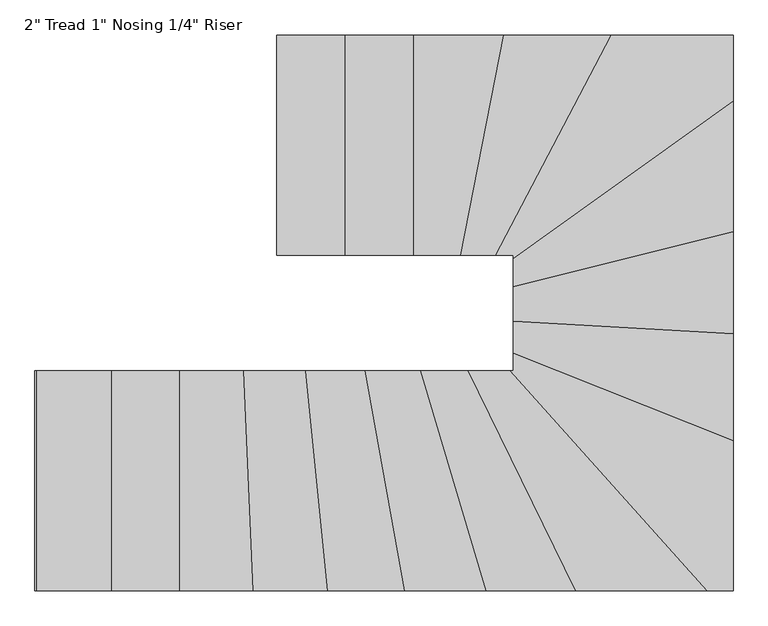
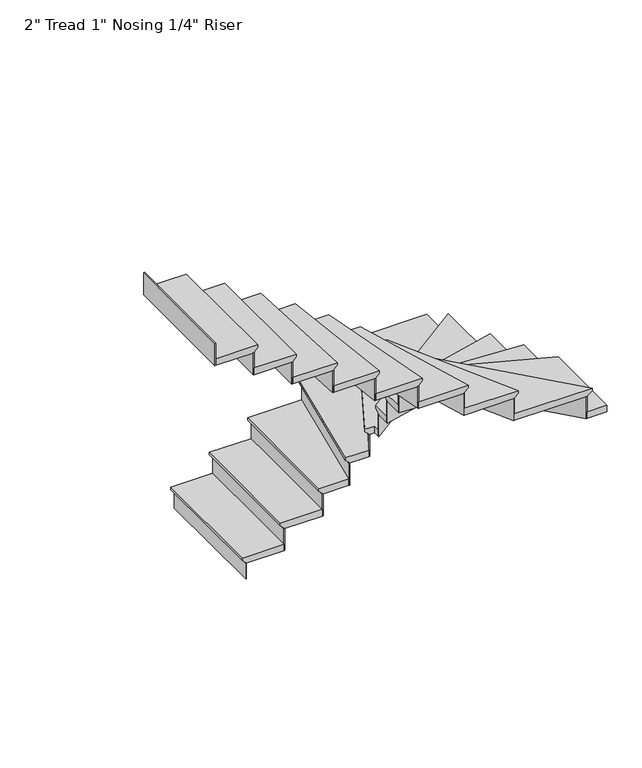
"""IFC4 building model written with IfcOpenShell, lengths in millimetres: stair flight geometry."""

from ifc_helpers import new_model, si_unit, origin, place, context, project, spatial, faceted_brep, source, transform, mapped, element, save


def stair_flight_f84afbbd(model_context):
    return source(origin(), model_context, "Body", "Brep", [
        faceted_brep([(158.6923968, 2024.0935985, 150.2833333), (158.6923968, 2024.0935985, 169.3333333), (158.6923968, 2922.8476133, 169.3333333), (158.6923968, 2922.8476133, 150.2833333), (184.0923968, 2024.0935985, 124.8833333), (184.0923968, 2922.8476133, 124.8833333), (463.4923968, 2024.0935985, 169.3333333), (463.4923968, 2922.8476133, 169.3333333), (184.0923968, 2922.8476133, 118.5333333), (463.4923968, 2922.8476133, 118.5333333), (463.4923968, 2024.0935985, 118.5333333), (184.0923968, 2024.0935985, 118.5333333)], [[[0, 1, 2, 3]], [[4, 0, 3, 5]], [[2, 1, 6, 7]], [[8, 9, 10, 11]], [[2, 7, 9, 8, 5, 3]], [[8, 11, 4, 5]], [[6, 1, 0, 4, 11, 10]], [[7, 6, 10, 9]]]),
        faceted_brep([(184.0923968, 2024.0935985, 118.5333333), (184.0923968, 2024.0935985, 0.0), (190.4423968, 2024.0935985, 0.0), (190.4423968, 2024.0935985, 118.5333333), (184.0923968, 2922.8476133, 118.5333333), (190.4423968, 2922.8476133, 118.5333333), (190.4423968, 2922.8476133, 0.0), (184.0923968, 2922.8476133, 0.0)], [[[0, 1, 2, 3]], [[4, 5, 6, 7]], [[1, 0, 4, 7]], [[2, 1, 7, 6]], [[3, 2, 6, 5]], [[0, 3, 5, 4]]]),
        faceted_brep([(463.4923968, 2024.0935985, 287.8666667), (463.4923968, 2024.0935985, 118.5333333), (469.8423968, 2024.0935985, 118.5333333), (469.8423968, 2024.0935985, 287.8666667), (463.4923968, 2922.8476133, 287.8666667), (469.8423968, 2922.8476133, 287.8666667), (469.8423968, 2922.8476133, 118.5333333), (463.4923968, 2922.8476133, 118.5333333)], [[[0, 1, 2, 3]], [[4, 5, 6, 7]], [[1, 0, 4, 7]], [[2, 1, 7, 6]], [[3, 2, 6, 5]], [[0, 3, 5, 4]]]),
        faceted_brep([(438.0923968, 2922.8476133, 338.6666667), (438.0923968, 2024.0935985, 338.6666667), (742.8923968, 2024.0935985, 338.6666667), (742.8923968, 2922.8476133, 338.6666667), (463.4923968, 2922.8476133, 287.8666667), (742.8923968, 2922.8476133, 287.8666667), (742.8923968, 2024.0935985, 287.8666667), (463.4923968, 2024.0935985, 287.8666667), (463.4923968, 2922.8476133, 294.2166667), (438.0923968, 2922.8476133, 319.6166667), (463.4923968, 2024.0935985, 294.2166667), (438.0923968, 2024.0935985, 319.6166667)], [[[0, 1, 2, 3]], [[4, 5, 6, 7]], [[0, 3, 5, 4, 8, 9]], [[4, 7, 10, 8]], [[2, 1, 11, 10, 7, 6]], [[3, 2, 6, 5]], [[11, 1, 0, 9]], [[10, 11, 9, 8]]]),
        faceted_brep([(742.8923968, 2024.0935985, 457.2), (742.8923968, 2024.0935985, 287.8666667), (749.2423968, 2024.0935985, 287.8666667), (749.2423968, 2024.0935985, 457.2), (742.8923968, 2922.8476133, 457.2), (749.2423968, 2922.8476133, 457.2), (749.2423968, 2922.8476133, 287.8666667), (742.8923968, 2922.8476133, 287.8666667)], [[[0, 1, 2, 3]], [[4, 5, 6, 7]], [[1, 0, 4, 7]], [[2, 1, 7, 6]], [[3, 2, 6, 5]], [[0, 3, 5, 4]]]),
        faceted_brep([(717.4923968, 2922.8476133, 508.0), (717.4923968, 2024.0935985, 508.0), (934.4682952, 2024.0935985, 508.0), (1111.0881205, 2922.8476133, 508.0), (742.8923968, 2922.8476133, 457.2), (1111.0881205, 2922.8476133, 457.2), (934.4682952, 2024.0935985, 457.2), (742.8923968, 2024.0935985, 457.2), (742.8923968, 2922.8476133, 463.55), (717.4923968, 2922.8476133, 488.95), (742.8923968, 2024.0935985, 463.55), (717.4923968, 2024.0935985, 488.95)], [[[0, 1, 2, 3]], [[4, 5, 6, 7]], [[0, 3, 5, 4, 8, 9]], [[4, 7, 10, 8]], [[2, 1, 11, 10, 7, 6]], [[3, 2, 6, 5]], [[11, 1, 0, 9]], [[10, 11, 9, 8]]]),
        faceted_brep([(934.4682952, 2024.0935985, 626.5333333), (934.4682952, 2024.0935985, 457.2), (940.939748, 2024.0935985, 457.2), (940.939748, 2024.0935985, 626.5333333), (1111.0881205, 2922.8476133, 626.5333333), (1117.5595733, 2922.8476133, 626.5333333), (1117.5595733, 2922.8476133, 457.2), (1111.0881205, 2922.8476133, 457.2)], [[[0, 1, 2, 3]], [[4, 5, 6, 7]], [[1, 0, 4, 7]], [[2, 1, 7, 6]], [[3, 2, 6, 5]], [[0, 3, 5, 4]]]),
        faceted_brep([(1085.2023094, 2922.8476133, 677.3333333), (908.5824841, 2024.0935985, 677.3333333), (1081.601446, 2024.0935985, 677.3333333), (1553.5566487, 2922.8476133, 677.3333333), (1111.0881205, 2922.8476133, 626.5333333), (1553.5566487, 2922.8476133, 626.5333333), (1081.601446, 2024.0935985, 626.5333333), (934.4682952, 2024.0935985, 626.5333333), (1111.0881205, 2922.8476133, 632.8833333), (1085.2023094, 2922.8476133, 658.2833333), (934.4682952, 2024.0935985, 632.8833333), (908.5824841, 2024.0935985, 658.2833333)], [[[0, 1, 2, 3]], [[4, 5, 6, 7]], [[0, 3, 5, 4, 8, 9]], [[4, 7, 10, 8]], [[2, 1, 11, 10, 7, 6]], [[3, 2, 6, 5]], [[11, 1, 0, 9]], [[10, 11, 9, 8]]]),
        faceted_brep([(1081.601446, 2024.0935985, 795.8666667), (1081.601446, 2024.0935985, 626.5333333), (1088.7737218, 2024.0935985, 626.5333333), (1088.7737218, 2024.0935985, 795.8666667), (1553.5566487, 2922.8476133, 795.8666667), (1560.7289245, 2922.8476133, 795.8666667), (1560.7289245, 2922.8476133, 626.5333333), (1553.5566487, 2922.8476133, 626.5333333)], [[[0, 1, 2, 3]], [[4, 5, 6, 7]], [[1, 0, 4, 7]], [[2, 1, 7, 6]], [[3, 2, 6, 5]], [[0, 3, 5, 4]]]),
        faceted_brep([(2022.1441983, 2621.1058304, 846.6666667), (2022.1441983, 2922.8476133, 846.6666667), (1524.8675453, 2922.8476133, 846.6666667), (1052.9123426, 2024.0935985, 846.6666667), (1123.3901835, 2024.0935985, 846.6666667), (1123.3901835, 1978.1363323, 846.6666667), (2022.1441983, 2922.8476133, 795.8666667), (2022.1441983, 2621.1058304, 795.8666667), (1123.3901835, 1978.1363323, 795.8666667), (1123.3901835, 2024.0935985, 795.8666667), (1081.601446, 2024.0935985, 795.8666667), (1553.5566487, 2922.8476133, 795.8666667), (1081.601446, 2024.0935985, 802.2166667), (1553.5566487, 2922.8476133, 802.2166667), (1052.9123426, 2024.0935985, 827.6166667), (1524.8675453, 2922.8476133, 827.6166667)], [[[0, 1, 2, 3, 4, 5]], [[6, 7, 8, 9, 10, 11]], [[1, 0, 7, 6]], [[11, 10, 12, 13]], [[4, 3, 14, 12, 10, 9]], [[0, 5, 8, 7]], [[14, 3, 2, 15]], [[12, 14, 15, 13]], [[5, 4, 9, 8]], [[2, 1, 6, 11, 13, 15]]]),
        faceted_brep([(1123.3901835, 1978.1363323, 965.2), (1123.3901835, 1978.1363323, 795.8666667), (1123.3901835, 1970.328676, 795.8666667), (1123.3901835, 1970.328676, 965.2), (2022.1441983, 2621.1058304, 965.2), (2022.1441983, 2613.298174, 965.2), (2022.1441983, 2613.298174, 795.8666667), (2022.1441983, 2621.1058304, 795.8666667)], [[[0, 1, 2, 3]], [[4, 5, 6, 7]], [[1, 0, 4, 7]], [[2, 1, 7, 6]], [[3, 2, 6, 5]], [[0, 3, 5, 4]]]),
        faceted_brep([(2022.1441983, 2652.3364556, 1016.0), (1123.3901835, 2009.3669576, 1016.0), (1123.3901835, 1868.1880985, 1016.0), (2022.1441983, 2093.75794, 1016.0), (2022.1441983, 2621.1058304, 965.2), (2022.1441983, 2093.75794, 965.2), (1123.3901835, 1868.1880985, 965.2), (1123.3901835, 1978.1363323, 965.2), (2022.1441983, 2621.1058304, 971.55), (2022.1441983, 2652.3364556, 996.95), (1123.3901835, 1978.1363323, 971.55), (1123.3901835, 2009.3669576, 996.95)], [[[0, 1, 2, 3]], [[4, 5, 6, 7]], [[0, 3, 5, 4, 8, 9]], [[4, 7, 10, 8]], [[2, 1, 11, 10, 7, 6]], [[3, 2, 6, 5]], [[11, 1, 0, 9]], [[10, 11, 9, 8]]]),
        faceted_brep([(1123.3901835, 1868.1880985, 1134.5333333), (1123.3901835, 1868.1880985, 965.2), (1123.3901835, 1861.6411553, 965.2), (1123.3901835, 1861.6411553, 1134.5333333), (2022.1441983, 2093.75794, 1134.5333333), (2022.1441983, 2087.2109968, 1134.5333333), (2022.1441983, 2087.2109968, 965.2), (2022.1441983, 2093.75794, 965.2)], [[[0, 1, 2, 3]], [[4, 5, 6, 7]], [[1, 0, 4, 7]], [[2, 1, 7, 6]], [[3, 2, 6, 5]], [[0, 3, 5, 4]]]),
        faceted_brep([(2022.1441983, 2119.9457129, 1185.3333333), (1123.3901835, 1894.3758714, 1185.3333333), (1123.3901835, 1727.7101185, 1185.3333333), (2022.1441983, 1676.930447, 1185.3333333), (2022.1441983, 2093.75794, 1134.5333333), (2022.1441983, 1676.930447, 1134.5333333), (1123.3901835, 1727.7101185, 1134.5333333), (1123.3901835, 1868.1880985, 1134.5333333), (2022.1441983, 2093.75794, 1140.8833333), (2022.1441983, 2119.9457129, 1166.2833333), (1123.3901835, 1868.1880985, 1140.8833333), (1123.3901835, 1894.3758714, 1166.2833333)], [[[0, 1, 2, 3]], [[4, 5, 6, 7]], [[0, 3, 5, 4, 8, 9]], [[4, 7, 10, 8]], [[2, 1, 11, 10, 7, 6]], [[3, 2, 6, 5]], [[11, 1, 0, 9]], [[10, 11, 9, 8]]]),
        faceted_brep([(1123.3901835, 1727.7101185, 1303.8666667), (1123.3901835, 1727.7101185, 1134.5333333), (1123.3901835, 1721.3499912, 1134.5333333), (1123.3901835, 1721.3499912, 1303.8666667), (2022.1441983, 1676.930447, 1303.8666667), (2022.1441983, 1670.5703197, 1303.8666667), (2022.1441983, 1670.5703197, 1134.5333333), (2022.1441983, 1676.930447, 1134.5333333)], [[[0, 1, 2, 3]], [[4, 5, 6, 7]], [[1, 0, 4, 7]], [[2, 1, 7, 6]], [[3, 2, 6, 5]], [[0, 3, 5, 4]]]),
        faceted_brep([(2022.1441983, 1702.3709564, 1354.6666667), (1123.3901835, 1753.1506279, 1354.6666667), (1123.3901835, 1594.7393557, 1354.6666667), (2022.1441983, 1238.4229709, 1354.6666667), (2022.1441983, 1676.930447, 1303.8666667), (2022.1441983, 1238.4229709, 1303.8666667), (1123.3901835, 1594.7393557, 1303.8666667), (1123.3901835, 1727.7101185, 1303.8666667), (2022.1441983, 1676.930447, 1310.2166667), (2022.1441983, 1702.3709564, 1335.6166667), (1123.3901835, 1727.7101185, 1310.2166667), (1123.3901835, 1753.1506279, 1335.6166667)], [[[0, 1, 2, 3]], [[4, 5, 6, 7]], [[0, 3, 5, 4, 8, 9]], [[4, 7, 10, 8]], [[3, 2, 6, 5]], [[11, 1, 0, 9]], [[10, 11, 9, 8]], [[2, 1, 11, 10, 7, 6]]]),
        faceted_brep([(1123.3901835, 1594.7393557, 1473.2), (1123.3901835, 1594.7393557, 1303.8666667), (1123.3901835, 1587.9085225, 1303.8666667), (1123.3901835, 1587.9085225, 1473.2), (2022.1441983, 1238.4229709, 1473.2), (2022.1441983, 1231.5921376, 1473.2), (2022.1441983, 1231.5921376, 1303.8666667), (2022.1441983, 1238.4229709, 1303.8666667)], [[[0, 1, 2, 3]], [[4, 5, 6, 7]], [[1, 0, 4, 7]], [[2, 1, 7, 6]], [[3, 2, 6, 5]], [[0, 3, 5, 4]]]),
        faceted_brep([(1880.1651285, 652.4935985, 1524.0), (2022.1441983, 652.4935985, 1524.0), (2022.1441983, 1265.7463038, 1524.0), (1123.3901835, 1622.0626887, 1524.0), (1123.3901835, 1551.2476133, 1524.0), (1076.3040211, 1551.2476133, 1524.0), (2022.1441983, 652.4935985, 1473.2), (1880.1651285, 652.4935985, 1473.2), (1076.3040211, 1551.2476133, 1473.2), (1123.3901835, 1551.2476133, 1473.2), (1123.3901835, 1594.7393557, 1473.2), (2022.1441983, 1238.4229709, 1473.2), (1123.3901835, 1594.7393557, 1479.55), (2022.1441983, 1238.4229709, 1479.55), (1123.3901835, 1622.0626887, 1504.95), (2022.1441983, 1265.7463038, 1504.95)], [[[0, 1, 2, 3, 4, 5]], [[6, 7, 8, 9, 10, 11]], [[1, 0, 7, 6]], [[11, 10, 12, 13]], [[4, 3, 14, 12, 10, 9]], [[0, 5, 8, 7]], [[14, 3, 2, 15]], [[12, 14, 15, 13]], [[2, 1, 6, 11, 13, 15]], [[5, 4, 9, 8]]]),
        faceted_brep([(1076.3040211, 1551.2476133, 1642.5333333), (1076.3040211, 1551.2476133, 1473.2), (1067.7846442, 1551.2476133, 1473.2), (1067.7846442, 1551.2476133, 1642.5333333), (1880.1651285, 652.4935985, 1642.5333333), (1871.6457515, 652.4935985, 1642.5333333), (1871.6457515, 652.4935985, 1473.2), (1880.1651285, 652.4935985, 1473.2)], [[[0, 1, 2, 3]], [[4, 5, 6, 7]], [[1, 0, 4, 7]], [[2, 1, 7, 6]], [[3, 2, 6, 5]], [[0, 3, 5, 4]]]),
        faceted_brep([(1914.2426364, 652.4935985, 1693.3333333), (1110.381529, 1551.2476133, 1693.3333333), (909.9761874, 1551.2476133, 1693.3333333), (1349.6820711, 652.4935985, 1693.3333333), (1880.1651285, 652.4935985, 1642.5333333), (1349.6820711, 652.4935985, 1642.5333333), (909.9761874, 1551.2476133, 1642.5333333), (1076.3040211, 1551.2476133, 1642.5333333), (1880.1651285, 652.4935985, 1648.8833333), (1914.2426364, 652.4935985, 1674.2833333), (1076.3040211, 1551.2476133, 1648.8833333), (1110.381529, 1551.2476133, 1674.2833333)], [[[0, 1, 2, 3]], [[4, 5, 6, 7]], [[0, 3, 5, 4, 8, 9]], [[4, 7, 10, 8]], [[2, 1, 11, 10, 7, 6]], [[3, 2, 6, 5]], [[11, 1, 0, 9]], [[10, 11, 9, 8]]]),
        faceted_brep([(909.9761874, 1551.2476133, 1811.8666667), (909.9761874, 1551.2476133, 1642.5333333), (902.9069653, 1551.2476133, 1642.5333333), (902.9069653, 1551.2476133, 1811.8666667), (1349.6820711, 652.4935985, 1811.8666667), (1342.6128491, 652.4935985, 1811.8666667), (1342.6128491, 652.4935985, 1642.5333333), (1349.6820711, 652.4935985, 1642.5333333)], [[[0, 1, 2, 3]], [[4, 5, 6, 7]], [[1, 0, 4, 7]], [[2, 1, 7, 6]], [[3, 2, 6, 5]], [[0, 3, 5, 4]]]),
        faceted_brep([(1377.9589592, 652.4935985, 1862.6666667), (938.2530755, 1551.2476133, 1862.6666667), (717.8211109, 1551.2476133, 1862.6666667), (985.3279709, 652.4935985, 1862.6666667), (1349.6820711, 652.4935985, 1811.8666667), (985.3279709, 652.4935985, 1811.8666667), (717.8211109, 1551.2476133, 1811.8666667), (909.9761874, 1551.2476133, 1811.8666667), (1349.6820711, 652.4935985, 1818.2166667), (1377.9589592, 652.4935985, 1843.6166667), (909.9761874, 1551.2476133, 1818.2166667), (938.2530755, 1551.2476133, 1843.6166667)], [[[0, 1, 2, 3]], [[4, 5, 6, 7]], [[0, 3, 5, 4, 8, 9]], [[4, 7, 10, 8]], [[2, 1, 11, 10, 7, 6]], [[3, 2, 6, 5]], [[11, 1, 0, 9]], [[10, 11, 9, 8]]]),
        faceted_brep([(717.8211109, 1551.2476133, 1981.2), (717.8211109, 1551.2476133, 1811.8666667), (711.1958034, 1551.2476133, 1811.8666667), (711.1958034, 1551.2476133, 1981.2), (985.3279709, 652.4935985, 1981.2), (978.7026634, 652.4935985, 1981.2), (978.7026634, 652.4935985, 1811.8666667), (985.3279709, 652.4935985, 1811.8666667)], [[[0, 1, 2, 3]], [[4, 5, 6, 7]], [[1, 0, 4, 7]], [[2, 1, 7, 6]], [[3, 2, 6, 5]], [[0, 3, 5, 4]]]),
        faceted_brep([(1011.8292006, 652.4935985, 2032.0), (744.3223406, 1551.2476133, 2032.0), (491.9145253, 1551.2476133, 2032.0), (653.8193232, 652.4935985, 2032.0), (985.3279709, 652.4935985, 1981.2), (653.8193232, 652.4935985, 1981.2), (491.9145253, 1551.2476133, 1981.2), (717.8211109, 1551.2476133, 1981.2), (985.3279709, 652.4935985, 1987.55), (1011.8292006, 652.4935985, 2012.95), (717.8211109, 1551.2476133, 1987.55), (744.3223406, 1551.2476133, 2012.95)], [[[0, 1, 2, 3]], [[4, 5, 6, 7]], [[0, 3, 5, 4, 8, 9]], [[4, 7, 10, 8]], [[2, 1, 11, 10, 7, 6]], [[3, 2, 6, 5]], [[11, 1, 0, 9]], [[10, 11, 9, 8]]]),
        faceted_brep([(491.9145253, 1551.2476133, 2150.5333333), (491.9145253, 1551.2476133, 1981.2), (485.4623137, 1551.2476133, 1981.2), (485.4623137, 1551.2476133, 2150.5333333), (653.8193232, 652.4935985, 2150.5333333), (647.3671116, 652.4935985, 2150.5333333), (647.3671116, 652.4935985, 1981.2), (653.8193232, 652.4935985, 1981.2)], [[[0, 1, 2, 3]], [[4, 5, 6, 7]], [[1, 0, 4, 7]], [[2, 1, 7, 6]], [[3, 2, 6, 5]], [[0, 3, 5, 4]]]),
        faceted_brep([(679.6281696, 652.4935985, 2201.3333333), (517.7233717, 1551.2476133, 2201.3333333), (248.510664, 1551.2476133, 2201.3333333), (338.9841344, 652.4935985, 2201.3333333), (653.8193232, 652.4935985, 2150.5333333), (338.9841344, 652.4935985, 2150.5333333), (248.510664, 1551.2476133, 2150.5333333), (491.9145253, 1551.2476133, 2150.5333333), (653.8193232, 652.4935985, 2156.8833333), (679.6281696, 652.4935985, 2182.2833333), (491.9145253, 1551.2476133, 2156.8833333), (517.7233717, 1551.2476133, 2182.2833333)], [[[0, 1, 2, 3]], [[4, 5, 6, 7]], [[0, 3, 5, 4, 8, 9]], [[4, 7, 10, 8]], [[2, 1, 11, 10, 7, 6]], [[3, 2, 6, 5]], [[11, 1, 0, 9]], [[10, 11, 9, 8]]]),
        faceted_brep([(248.510664, 1551.2476133, 2319.8666667), (248.510664, 1551.2476133, 2150.5333333), (242.1285711, 1551.2476133, 2150.5333333), (242.1285711, 1551.2476133, 2319.8666667), (338.9841344, 652.4935985, 2319.8666667), (332.6020415, 652.4935985, 2319.8666667), (332.6020415, 652.4935985, 2150.5333333), (338.9841344, 652.4935985, 2150.5333333)], [[[0, 1, 2, 3]], [[4, 5, 6, 7]], [[1, 0, 4, 7]], [[2, 1, 7, 6]], [[3, 2, 6, 5]], [[0, 3, 5, 4]]]),
        faceted_brep([(364.5125059, 652.4935985, 2370.6666667), (274.0390354, 1551.2476133, 2370.6666667), (-5.0166043, 1551.2476133, 2370.6666667), (33.9204942, 652.4935985, 2370.6666667), (338.9841344, 652.4935985, 2319.8666667), (33.9204942, 652.4935985, 2319.8666667), (-5.0166043, 1551.2476133, 2319.8666667), (248.510664, 1551.2476133, 2319.8666667), (338.9841344, 652.4935985, 2326.2166667), (364.5125059, 652.4935985, 2351.6166667), (248.510664, 1551.2476133, 2326.2166667), (274.0390354, 1551.2476133, 2351.6166667)], [[[0, 1, 2, 3]], [[4, 5, 6, 7]], [[0, 3, 5, 4, 8, 9]], [[4, 7, 10, 8]], [[2, 1, 11, 10, 7, 6]], [[3, 2, 6, 5]], [[11, 1, 0, 9]], [[10, 11, 9, 8]]]),
        faceted_brep([(-5.0166043, 1551.2476133, 2489.2), (-5.0166043, 1551.2476133, 2319.8666667), (-11.3725607, 1551.2476133, 2319.8666667), (-11.3725607, 1551.2476133, 2489.2), (33.9204942, 652.4935985, 2489.2), (27.5645378, 652.4935985, 2489.2), (27.5645378, 652.4935985, 2319.8666667), (33.9204942, 652.4935985, 2319.8666667)], [[[0, 1, 2, 3]], [[4, 5, 6, 7]], [[1, 0, 4, 7]], [[2, 1, 7, 6]], [[3, 2, 6, 5]], [[0, 3, 5, 4]]]),
        faceted_brep([(59.3443199, 652.4935985, 2540.0), (20.4072214, 1551.2476133, 2540.0), (-264.9242294, 1551.2476133, 2540.0), (-264.9242294, 652.4935985, 2540.0), (33.9204942, 652.4935985, 2489.2), (-264.9242294, 652.4935985, 2489.2), (-264.9242294, 1551.2476133, 2489.2), (-5.0166043, 1551.2476133, 2489.2), (33.9204942, 652.4935985, 2495.55), (59.3443199, 652.4935985, 2520.95), (-5.0166043, 1551.2476133, 2495.55), (20.4072214, 1551.2476133, 2520.95)], [[[0, 1, 2, 3]], [[4, 5, 6, 7]], [[0, 3, 5, 4, 8, 9]], [[4, 7, 10, 8]], [[2, 1, 11, 10, 7, 6]], [[3, 2, 6, 5]], [[11, 1, 0, 9]], [[10, 11, 9, 8]]]),
        faceted_brep([(-264.9242294, 1551.2476133, 2658.5333333), (-264.9242294, 1551.2476133, 2489.2), (-271.2742294, 1551.2476133, 2489.2), (-271.2742294, 1551.2476133, 2658.5333333), (-264.9242294, 652.4935985, 2658.5333333), (-271.2742294, 652.4935985, 2658.5333333), (-271.2742294, 652.4935985, 2489.2), (-264.9242294, 652.4935985, 2489.2)], [[[0, 1, 2, 3]], [[4, 5, 6, 7]], [[1, 0, 4, 7]], [[2, 1, 7, 6]], [[3, 2, 6, 5]], [[0, 3, 5, 4]]]),
        faceted_brep([(-239.5242294, 652.4935985, 2709.3333333), (-239.5242294, 1551.2476133, 2709.3333333), (-544.3242294, 1551.2476133, 2709.3333333), (-544.3242294, 652.4935985, 2709.3333333), (-264.9242294, 652.4935985, 2658.5333333), (-544.3242294, 652.4935985, 2658.5333333), (-544.3242294, 1551.2476133, 2658.5333333), (-264.9242294, 1551.2476133, 2658.5333333), (-264.9242294, 652.4935985, 2664.8833333), (-239.5242294, 652.4935985, 2690.2833333), (-264.9242294, 1551.2476133, 2664.8833333), (-239.5242294, 1551.2476133, 2690.2833333)], [[[0, 1, 2, 3]], [[4, 5, 6, 7]], [[0, 3, 5, 4, 8, 9]], [[4, 7, 10, 8]], [[2, 1, 11, 10, 7, 6]], [[3, 2, 6, 5]], [[11, 1, 0, 9]], [[10, 11, 9, 8]]]),
        faceted_brep([(-544.3242294, 1551.2476133, 2827.8666667), (-544.3242294, 1551.2476133, 2658.5333333), (-550.6742294, 1551.2476133, 2658.5333333), (-550.6742294, 1551.2476133, 2827.8666667), (-544.3242294, 652.4935985, 2827.8666667), (-550.6742294, 652.4935985, 2827.8666667), (-550.6742294, 652.4935985, 2658.5333333), (-544.3242294, 652.4935985, 2658.5333333)], [[[0, 1, 2, 3]], [[4, 5, 6, 7]], [[1, 0, 4, 7]], [[2, 1, 7, 6]], [[3, 2, 6, 5]], [[0, 3, 5, 4]]]),
        faceted_brep([(-823.7242294, 1551.2476133, 2997.2), (-823.7242294, 1551.2476133, 2827.8666667), (-830.0742294, 1551.2476133, 2827.8666667), (-830.0742294, 1551.2476133, 2997.2), (-823.7242294, 652.4935985, 2997.2), (-830.0742294, 652.4935985, 2997.2), (-830.0742294, 652.4935985, 2827.8666667), (-823.7242294, 652.4935985, 2827.8666667)], [[[0, 1, 2, 3]], [[4, 5, 6, 7]], [[1, 0, 4, 7]], [[2, 1, 7, 6]], [[3, 2, 6, 5]], [[0, 3, 5, 4]]]),
        faceted_brep([(-518.9242294, 652.4935985, 2878.6666667), (-518.9242294, 1551.2476133, 2878.6666667), (-823.7242294, 1551.2476133, 2878.6666667), (-823.7242294, 652.4935985, 2878.6666667), (-544.3242294, 652.4935985, 2827.8666667), (-823.7242294, 652.4935985, 2827.8666667), (-823.7242294, 1551.2476133, 2827.8666667), (-544.3242294, 1551.2476133, 2827.8666667), (-544.3242294, 652.4935985, 2834.2166667), (-518.9242294, 652.4935985, 2859.6166667), (-544.3242294, 1551.2476133, 2834.2166667), (-518.9242294, 1551.2476133, 2859.6166667)], [[[0, 1, 2, 3]], [[4, 5, 6, 7]], [[0, 3, 5, 4, 8, 9]], [[4, 7, 10, 8]], [[2, 1, 11, 10, 7, 6]], [[3, 2, 6, 5]], [[11, 1, 0, 9]], [[10, 11, 9, 8]]]),
    ])


if __name__ == "__main__":
    model = new_model("IFC4")
    model_context = context("Model", 3, world=origin())
    ifc_project = project(units=[si_unit("LENGTHUNIT", "METRE", prefix="MILLI")], contexts=[model_context])
    site = spatial("IfcSite", under=ifc_project)
    building = spatial("IfcBuilding", under=site)
    placement = place(None, origin())
    stair_flight_shape = stair_flight_f84afbbd(model_context)
    element("IfcStairFlight", 1, ObjectType="2\" Tread 1\" Nosing 1/4\" Riser", at=placement, inside=building, context=model_context, shape_type="MappedRepresentation", body=[
        mapped(stair_flight_shape, transform((0.0, 0.0, 0.0), x_axis=(1.0, 0.0, 0.0), y_axis=(0.0, 1.0, 0.0), z_axis=(0.0, 0.0, 1.0))),
    ])
    save(model, "model.ifc")
